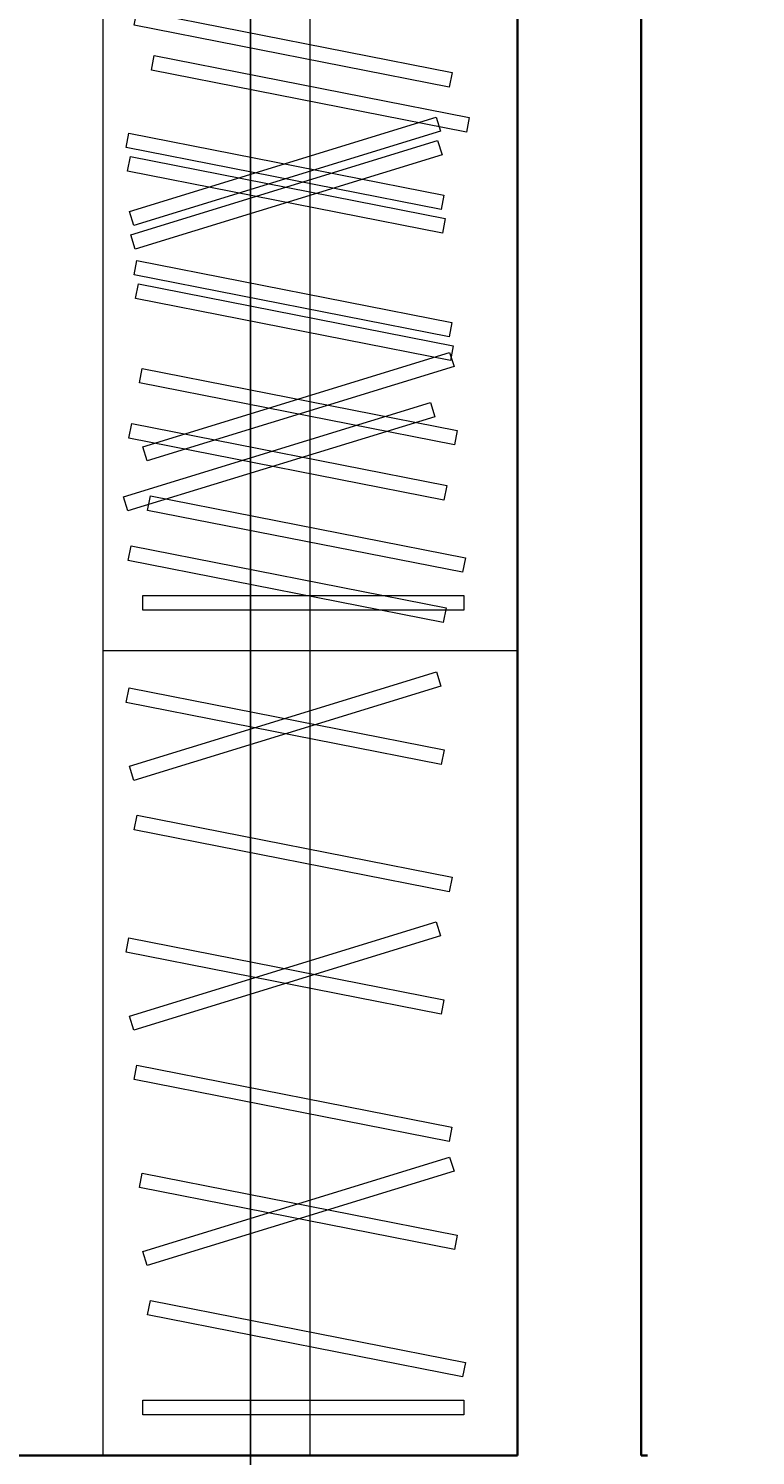
# Model space of a CAD drawing. Units: inches. Extents: x -61 to 1599, y -1316 to 257.
# Tile 64 of 204: x 205 to 240, y -282 to -213. Entities that reach past the tile are written whole.
import ezdxf

# ---------------------------------------------------------------- set-up
doc = ezdxf.new("R2010")
doc.units = ezdxf.units.IN
doc.header["$MEASUREMENT"] = 0
for name, color, linetype, lineweight in [('A-ANNO-DIMS', 2, 'Continuous', 18), ('A-FLOR-CASE', 8, 'Continuous', 18), ('WALLS', 4, 'Continuous', 35)]:
    doc.layers.add(name, color=color, linetype=linetype, lineweight=lineweight)
doc.styles.get("Standard").update_dxf_attribs({"font": 'arial.ttf'})
doc.dimstyles.get("Standard").update_dxf_attribs({"dimtxt": 0.18, "dimasz": 0.18, "dimexe": 0.18, "dimexo": 0.0625, "dimgap": 0.09, "dimtad": 0, "dimtih": 1, "dimtoh": 1, "dimdec": 0, "dimzin": 0, "dimdsep": 46, "dimlunit": 3, "dimtxsty": 'Standard', "dimcen": 0.09, "dimadec": 0, "dimazin": 0, "dimtfac": 1, "dimtdec": 0, "dimtofl": 0, "dimtmove": 0, "dimatfit": 3, "dimfxl": 1, "dimtolj": 1, "dimtzin": 0, "dimarcsym": 0})

# ---------------------------------------------------------------- blocks, each defined once
blk = doc.blocks.new('WARDROBE-HANGING')
blk.add_line((10.047, 0), (10.047, 68))
for points in [[(20.094, 0), (0, 0), (0, 68), (20.094, 68)], [(2.482, 67.852), (17.751, 64.849), (17.612, 64.142), (2.343, 67.146)], [(1.346, 59.162), (16.221, 63.731), (16.432, 63.043), (1.557, 58.474)], [(1.325, 62.957), (16.593, 59.954), (16.454, 59.247), (1.186, 62.251)], [(1.713, 56.784), (16.981, 53.781), (16.842, 53.074), (1.574, 56.078)], [(0.997, 46.467), (15.872, 51.036), (16.084, 50.348), (1.209, 45.779)], [(1.394, 50.014), (16.662, 47.011), (16.523, 46.305), (1.255, 49.308)], [(1.365, 44.09), (16.633, 41.086), (16.494, 40.38), (1.226, 43.383)], [(1.283, 33.408), (16.158, 37.977), (16.37, 37.289), (1.495, 32.72)], [(1.262, 37.203), (16.53, 34.2), (16.391, 33.493), (1.123, 36.497)], [(1.651, 31.03), (16.919, 28.027), (16.78, 27.32), (1.512, 30.324)], [(1.279, 21.299), (16.154, 25.868), (16.365, 25.18), (1.49, 20.611)], [(1.257, 25.094), (16.525, 22.091), (16.386, 21.384), (1.118, 24.388)], [(1.646, 18.921), (16.914, 15.918), (16.775, 15.211), (1.507, 18.215)], [(1.928, 9.892), (16.803, 14.461), (17.014, 13.773), (2.139, 9.203)], [(1.906, 13.687), (17.174, 10.684), (17.035, 9.977), (1.767, 12.981)], [(2.295, 7.514), (17.563, 4.511), (17.424, 3.804), (2.156, 6.808)], [(17.491, 1.962), (1.93, 1.962), (1.93, 2.682), (17.491, 2.682)]]:
    blk.add_lwpolyline(points, close=True)
blk = doc.blocks.new('WARDROBE-HANGING-3')
blk.add_line((10.047, 0), (10.047, 68))
blk.add_lwpolyline([(20.094, 68), (20.094, 68), (20.094, 0), (0, 0), (0, 68)])
for points in [[(2.482, 67.852), (17.751, 64.849), (17.612, 64.142), (2.343, 67.146)], [(1.346, 59.162), (16.221, 63.731), (16.432, 63.043), (1.557, 58.474)], [(1.325, 62.957), (16.593, 59.954), (16.454, 59.247), (1.186, 62.251)], [(1.713, 56.784), (16.981, 53.781), (16.842, 53.074), (1.574, 56.078)], [(0.997, 46.467), (15.872, 51.036), (16.084, 50.348), (1.209, 45.779)], [(1.394, 50.014), (16.662, 47.011), (16.523, 46.305), (1.255, 49.308)], [(1.365, 44.09), (16.633, 41.086), (16.494, 40.38), (1.226, 43.383)], [(1.283, 33.408), (16.158, 37.977), (16.37, 37.289), (1.495, 32.72)], [(1.262, 37.203), (16.53, 34.2), (16.391, 33.493), (1.123, 36.497)], [(1.651, 31.03), (16.919, 28.027), (16.78, 27.32), (1.512, 30.324)], [(1.279, 21.299), (16.154, 25.868), (16.365, 25.18), (1.49, 20.611)], [(1.257, 25.094), (16.525, 22.091), (16.386, 21.384), (1.118, 24.388)], [(1.646, 18.921), (16.914, 15.918), (16.775, 15.211), (1.507, 18.215)], [(1.928, 9.892), (16.803, 14.461), (17.014, 13.773), (2.139, 9.203)], [(1.906, 13.687), (17.174, 10.684), (17.035, 9.977), (1.767, 12.981)], [(2.295, 7.514), (17.563, 4.511), (17.424, 3.804), (2.156, 6.808)], [(17.491, 1.962), (1.93, 1.962), (1.93, 2.682), (17.491, 2.682)]]:
    blk.add_lwpolyline(points, close=True)
blk = doc.blocks.new('*D687')
at = {"layer": 'A-ANNO-DIMS', "color": 0, "lineweight": -2, "transparency": 16777216}
for p, q in [((289.418, 181.677), (-61.077, 181.677)), ((-60.897, 181.497), (-60.897, -528.952)), ((-60.897, -1239.765), (-60.897, -529.316)), ((319.64, -1239.945), (-61.077, -1239.945))]:
    blk.add_line(p, q, dxfattribs=at)
at = {"layer": 'A-ANNO-DIMS', "color": 0, "transparency": 16777216}
for points in [[(-60.927, 181.497), (-60.867, 181.497), (-60.897, 181.677)], [(-60.927, -1239.765), (-60.867, -1239.765), (-60.897, -1239.945)]]:
    blk.add_solid(points, dxfattribs=at)
at = {"layer": 'DEFPOINTS', "color": 0, "transparency": 16777216}
for p in [(289.481, 181.677), (-60.897, -1239.945), (319.703, -1239.945)]:
    blk.add_point(p, dxfattribs=at)
at = {"layer": 'A-ANNO-DIMS', "color": 0, "transparency": 16777216, "insert": (-60.897, -529.134), "char_height": 0.18, "attachment_point": 5}
blk.add_mtext('\\A1;1421.6', dxfattribs=at)
blk = doc.blocks.new('*D699')
at = {"layer": 'A-ANNO-DIMS', "color": 0, "lineweight": -2, "transparency": 16777216}
for p, q in [((835.64, -167.169), (-61.077, -167.169)), ((-60.897, -167.349), (-60.897, -306.726)), ((-60.897, -446.466), (-60.897, -307.09)), ((841.64, -446.646), (-61.077, -446.646))]:
    blk.add_line(p, q, dxfattribs=at)
at = {"layer": 'A-ANNO-DIMS', "color": 0, "transparency": 16777216}
for points in [[(-60.927, -167.349), (-60.867, -167.349), (-60.897, -167.169)], [(-60.927, -446.466), (-60.867, -446.466), (-60.897, -446.646)]]:
    blk.add_solid(points, dxfattribs=at)
at = {"layer": 'DEFPOINTS', "color": 0, "transparency": 16777216}
for p in [(835.703, -167.169), (-60.897, -446.646), (841.703, -446.646)]:
    blk.add_point(p, dxfattribs=at)
at = {"layer": 'A-ANNO-DIMS', "color": 0, "transparency": 16777216, "insert": (-60.897, -306.908), "char_height": 0.18, "attachment_point": 5}
blk.add_mtext('\\A1;279.5', dxfattribs=at)
blk = doc.blocks.new('*D701')
at = {"layer": 'A-ANNO-DIMS', "color": 0, "lineweight": -2, "transparency": 16777216}
for p, q in [((215.752, -616.882), (215.752, 257.457)), ((215.932, 257.277), (233.924, 257.277)), ((252.702, 257.277), (234.711, 257.277)), ((252.882, -616.882), (252.882, 257.457))]:
    blk.add_line(p, q, dxfattribs=at)
at = {"layer": 'A-ANNO-DIMS', "color": 0, "transparency": 16777216}
for points in [[(215.932, 257.307), (215.932, 257.247), (215.752, 257.277)], [(252.702, 257.307), (252.702, 257.247), (252.882, 257.277)]]:
    blk.add_solid(points, dxfattribs=at)
at = {"layer": 'DEFPOINTS', "color": 0, "transparency": 16777216}
for p in [(252.882, 257.277), (215.752, -616.945), (252.882, -616.945)]:
    blk.add_point(p, dxfattribs=at)
at = {"layer": 'A-ANNO-DIMS', "color": 0, "transparency": 16777216, "insert": (234.317, 257.277), "char_height": 0.18, "attachment_point": 5}
blk.add_mtext('\\A1;37.13', dxfattribs=at)

msp = doc.modelspace()

# ---------------------------------------------------------------- linework, layer by layer
at = {"layer": 'WALLS'}
for p, q in [((234.7028, -282.3229), (234.7028, -169.3229)), ((228.7028, -282.3229), (228.7028, -175.3229)), ((165.7028, -282.3229), (228.7028, -282.3229)), ((234.7028, -282.3229), (234.999, -282.3229))]:
    msp.add_line(p, q, dxfattribs=at)

# ---------------------------------------------------------------- block references
at = {"layer": 'A-FLOR-CASE'}
for name, p in [('WARDROBE-HANGING', (208.609, -243.323)), ('WARDROBE-HANGING-3', (208.609, -282.323))]:
    msp.add_blockref(name, p, dxfattribs=at)

# ---------------------------------------------------------------- dimensions: what is measured, and where the dimension line sits
at = {"layer": 'A-ANNO-DIMS'}
dim = msp.add_linear_dim(base=(252.8825, 257.2771), p1=(215.7521, -616.9446), p2=(252.8825, -616.9446), dimstyle='Standard', override={"dimdec": 2, "dimlfac": 1, "dimrnd": 0, "dimzin": 0, "dimdsep": 46, "dimlunit": 2}, dxfattribs=at)
dim.commit()
dim.dimension.update_dxf_attribs({"geometry": '*D701', "text_midpoint": (234.3173, 257.2771)})
for base, p1, p2, picture, middle in [((-60.8972, -1239.9446), (289.4807, 181.6771), (319.7028, -1239.9446), '*D687', (-60.8972, -529.1337)), ((-60.8972, -446.6462), (835.7028, -167.169), (841.7028, -446.6462), '*D699', (-60.8972, -306.9076))]:
    dim = msp.add_linear_dim(base=base, p1=p1, p2=p2, angle=90, dimstyle='Standard', override={"dimdec": 1, "dimlfac": 1, "dimrnd": 0, "dimzin": 0, "dimdsep": 46, "dimlunit": 2}, dxfattribs=at)
    dim.commit()
    dim.dimension.update_dxf_attribs({"geometry": picture, "text_midpoint": middle})

doc.saveas('drawing.dxf')
